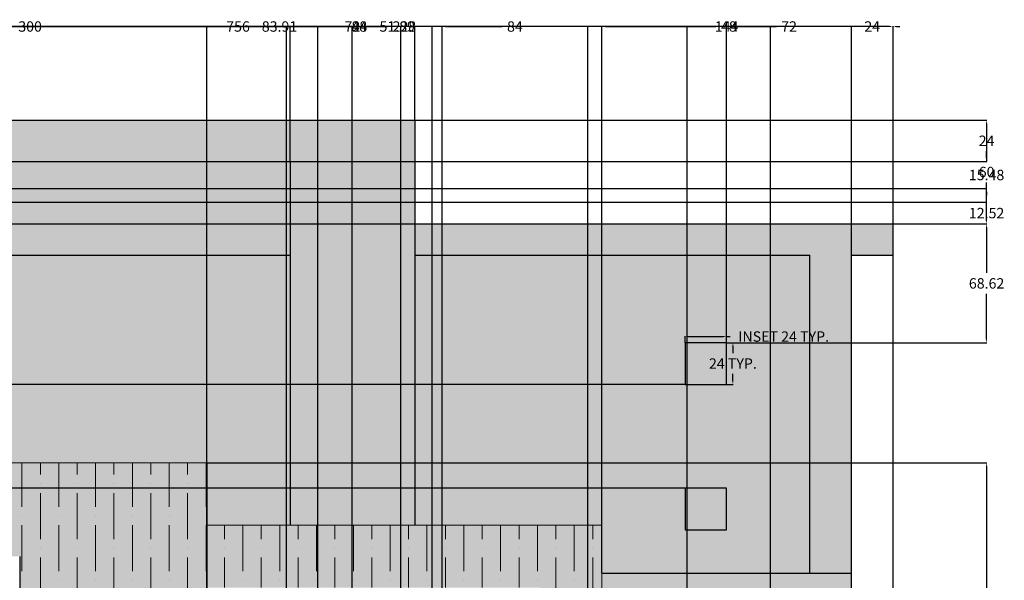
# Model space of a CAD drawing. Units: inches. Extents: x 180 to 1069, y 71 to 1267.
# Tile 8 of 8: x 498 to 1066, y 943 to 1267. Entities that reach past the tile are written whole.
import ezdxf

# ---------------------------------------------------------------- set-up
doc = ezdxf.new("R2010")
doc.units = ezdxf.units.IN
doc.header["$MEASUREMENT"] = 0
for name, color, linetype, lineweight in [('A-ANNO-DIMS', 2, 'Continuous', 18), ('A-ELEV-FRAM', 7, 'Continuous', 25), ('A-WALL', 7, 'Continuous', 30), ('A-WALL-CLAD', 7, 'Continuous', 18), ('A-WALL-SCRN-JNTS-PATT', 8, 'Continuous', 13)]:
    doc.layers.add(name, color=color, linetype=linetype, lineweight=lineweight)
for name, color, linetype, lineweight, true_color in [('A-ELEV-BAND-PATT', 30, 'Continuous', 13, 0xf26722), ('A-ELEV-FRAM-PATT', 53, 'Continuous', 13, 0xefd648), ('A-ELEV-REVL-PATT', 9, 'Continuous', 13, 0xc7c8ca), ('A-ELEV-TRIM-PATT', 7, 'Continuous', 13, 0xffffff), ('A-WALL-PATT', 253, 'Continuous', 13, 0x9f9f8e), ('A-WALL-SCRN-PATT', 251, 'Continuous', 13, 0x636466), ('A-WALL-STUC-PATT', 9, 'Continuous', 13, 0xc7c8ca)]:
    doc.layers.add(name, color=color, linetype=linetype, lineweight=lineweight, true_color=true_color)
doc.styles.get("Standard").update_dxf_attribs({"font": 'arial.ttf'})
doc.dimstyles.get("Standard").update_dxf_attribs({"dimtxt": 6, "dimasz": 2, "dimexe": 0.18, "dimexo": 0.0625, "dimgap": 3, "dimtad": 0, "dimtih": 1, "dimtoh": 1, "dimdec": 0, "dimzin": 0, "dimdsep": 46, "dimlunit": 3, "dimtxsty": 'Standard', "dimcen": 0.09, "dimadec": 0, "dimazin": 0, "dimtfac": 1, "dimtdec": 0, "dimtofl": 0, "dimtmove": 0, "dimatfit": 3, "dimfxl": 1, "dimtolj": 1, "dimtzin": 0, "dimarcsym": 0})

# ---------------------------------------------------------------- blocks, each defined once
blk = doc.blocks.new('FACADE-SQUARE-INSET')
blk.add_lwpolyline([(24, 24), (0, 24), (0, 0), (24, 0)], close=True)
blk = doc.blocks.new('*D6')
at = {"layer": 'A-ANNO-DIMS', "color": 0, "lineweight": -2, "transparency": 16777216}
for p, q in [((882.09, 1080.26), (882.09, 1083.98)), ((884.09, 1083.8), (904.09, 1083.8)), ((906.09, 1080.26), (906.09, 1083.98)), ((906.09, 1083.8), (908.09, 1083.8))]:
    blk.add_line(p, q, dxfattribs=at)
at = {"layer": 'A-ANNO-DIMS', "color": 0, "transparency": 16777216}
for points in [[(884.09, 1084.13), (884.09, 1083.47), (882.09, 1083.8)], [(904.09, 1084.13), (904.09, 1083.47), (906.09, 1083.8)]]:
    blk.add_solid(points, dxfattribs=at)
at = {"layer": 'Defpoints', "color": 0, "transparency": 16777216}
for p in [(882.09, 1080.2), (906.09, 1083.8), (906.09, 1080.2)]:
    blk.add_point(p, dxfattribs=at)
at = {"layer": 'A-ANNO-DIMS', "color": 0, "transparency": 16777216, "insert": (938.98, 1083.8), "char_height": 6, "attachment_point": 5}
blk.add_mtext('\\A1;INSET 24 TYP.', dxfattribs=at)
blk = doc.blocks.new('*D7')
at = {"layer": 'A-ANNO-DIMS', "color": 0, "lineweight": -2, "transparency": 16777216}
for p, q in [((906.15, 1080.2), (909.87, 1080.2)), ((909.69, 1078.2), (909.69, 1074.21)), ((909.69, 1058.2), (909.69, 1062.19)), ((906.15, 1056.2), (909.87, 1056.2))]:
    blk.add_line(p, q, dxfattribs=at)
at = {"layer": 'A-ANNO-DIMS', "color": 0, "transparency": 16777216}
for points in [[(909.35, 1078.2), (910.02, 1078.2), (909.69, 1080.2)], [(909.35, 1058.2), (910.02, 1058.2), (909.69, 1056.2)]]:
    blk.add_solid(points, dxfattribs=at)
at = {"layer": 'Defpoints', "color": 0, "transparency": 16777216}
for p in [(906.09, 1080.2), (906.09, 1056.2), (909.69, 1056.2)]:
    blk.add_point(p, dxfattribs=at)
at = {"layer": 'A-ANNO-DIMS', "color": 0, "transparency": 16777216, "insert": (909.69, 1068.2), "char_height": 6, "attachment_point": 5}
blk.add_mtext('\\A1;24 TYP.', dxfattribs=at)
blk = doc.blocks.new('*D16')
at = {"layer": 'A-ANNO-DIMS', "color": 0, "lineweight": -2, "transparency": 16777216}
for p, q in [((246.09, 1208.88), (246.09, 1263.01)), ((248.09, 1262.83), (614.49, 1262.83)), ((1000.09, 1262.83), (633.69, 1262.83)), ((1002.09, 1148.88), (1002.09, 1263.01))]:
    blk.add_line(p, q, dxfattribs=at)
at = {"layer": 'A-ANNO-DIMS', "color": 0, "transparency": 16777216}
for points in [[(248.09, 1263.16), (248.09, 1262.5), (246.09, 1262.83)], [(1000.09, 1263.16), (1000.09, 1262.5), (1002.09, 1262.83)]]:
    blk.add_solid(points, dxfattribs=at)
at = {"layer": 'Defpoints', "color": 0, "transparency": 16777216}
for p in [(1002.09, 1262.83), (246.09, 1208.82), (1002.09, 1148.82)]:
    blk.add_point(p, dxfattribs=at)
at = {"layer": 'A-ANNO-DIMS', "color": 0, "transparency": 16777216, "insert": (624.09, 1262.83), "char_height": 6, "attachment_point": 5}
blk.add_mtext('\\A1;756', dxfattribs=at)
blk = doc.blocks.new('*D18')
at = {"layer": 'A-ANNO-DIMS', "color": 0, "lineweight": -2, "transparency": 16777216}
for p, q in [((726.15, 1208.82), (1056.28, 1208.82)), ((1056.1, 1206.82), (1056.1, 1184.88)), ((1056.1, 1150.82), (1056.1, 1172.75)), ((1002.15, 1148.82), (1056.28, 1148.82))]:
    blk.add_line(p, q, dxfattribs=at)
at = {"layer": 'A-ANNO-DIMS', "color": 0, "transparency": 16777216}
for points in [[(1055.77, 1206.82), (1056.43, 1206.82), (1056.1, 1208.82)], [(1055.77, 1150.82), (1056.43, 1150.82), (1056.1, 1148.82)]]:
    blk.add_solid(points, dxfattribs=at)
at = {"layer": 'Defpoints', "color": 0, "transparency": 16777216}
for p in [(726.09, 1208.82), (1056.1, 1208.82), (1002.09, 1148.82)]:
    blk.add_point(p, dxfattribs=at)
at = {"layer": 'A-ANNO-DIMS', "color": 0, "transparency": 16777216, "insert": (1056.1, 1178.82), "char_height": 6, "attachment_point": 5}
blk.add_mtext('\\A1;60', dxfattribs=at)
blk = doc.blocks.new('*D21')
at = {"layer": 'A-ANNO-DIMS', "color": 0, "lineweight": -2, "transparency": 16777216}
for p, q in [((354.09, 1184.88), (354.09, 1263.01)), ((356.09, 1262.83), (494.47, 1262.83)), ((652.09, 1262.83), (513.7, 1262.83)), ((654.09, 1184.88), (654.09, 1263.01))]:
    blk.add_line(p, q, dxfattribs=at)
at = {"layer": 'A-ANNO-DIMS', "color": 0, "transparency": 16777216}
for points in [[(356.09, 1263.16), (356.09, 1262.5), (354.09, 1262.83)], [(652.09, 1263.16), (652.09, 1262.5), (654.09, 1262.83)]]:
    blk.add_solid(points, dxfattribs=at)
at = {"layer": 'Defpoints', "color": 0, "transparency": 16777216}
for p in [(654.09, 1262.83), (354.09, 1184.82), (654.09, 1184.82)]:
    blk.add_point(p, dxfattribs=at)
at = {"layer": 'A-ANNO-DIMS', "color": 0, "transparency": 16777216, "insert": (504.09, 1262.83), "char_height": 6, "attachment_point": 5}
blk.add_mtext('\\A1;300', dxfattribs=at)
blk = doc.blocks.new('*D22')
at = {"layer": 'A-ANNO-DIMS', "color": 0, "lineweight": -2, "transparency": 16777216}
for p, q in [((654.09, 1184.88), (654.09, 1263.01)), ((656.09, 1262.83), (682.85, 1262.83)), ((724.09, 1262.83), (697.33, 1262.83)), ((726.09, 1208.88), (726.09, 1263.01))]:
    blk.add_line(p, q, dxfattribs=at)
at = {"layer": 'A-ANNO-DIMS', "color": 0, "transparency": 16777216}
for points in [[(656.09, 1263.16), (656.09, 1262.5), (654.09, 1262.83)], [(724.09, 1263.16), (724.09, 1262.5), (726.09, 1262.83)]]:
    blk.add_solid(points, dxfattribs=at)
at = {"layer": 'Defpoints', "color": 0, "transparency": 16777216}
for p in [(726.09, 1262.83), (726.09, 1208.82), (654.09, 1184.82)]:
    blk.add_point(p, dxfattribs=at)
at = {"layer": 'A-ANNO-DIMS', "color": 0, "transparency": 16777216, "insert": (690.09, 1262.83), "char_height": 6, "attachment_point": 5}
blk.add_mtext('\\A1;72', dxfattribs=at)
blk = doc.blocks.new('*D23')
at = {"layer": 'A-ANNO-DIMS', "color": 0, "lineweight": -2, "transparency": 16777216}
for p, q in [((726.15, 1208.82), (1056.28, 1208.82)), ((1056.1, 1206.82), (1056.1, 1202.83)), ((1056.1, 1186.82), (1056.1, 1190.8)), ((654.15, 1184.82), (1056.28, 1184.82))]:
    blk.add_line(p, q, dxfattribs=at)
at = {"layer": 'A-ANNO-DIMS', "color": 0, "transparency": 16777216}
for points in [[(1055.77, 1206.82), (1056.43, 1206.82), (1056.1, 1208.82)], [(1055.77, 1186.82), (1056.43, 1186.82), (1056.1, 1184.82)]]:
    blk.add_solid(points, dxfattribs=at)
at = {"layer": 'Defpoints', "color": 0, "transparency": 16777216}
for p in [(726.09, 1208.82), (1056.1, 1208.82), (654.09, 1184.82)]:
    blk.add_point(p, dxfattribs=at)
at = {"layer": 'A-ANNO-DIMS', "color": 0, "transparency": 16777216, "insert": (1056.1, 1196.82), "char_height": 6, "attachment_point": 5}
blk.add_mtext('\\A1;24', dxfattribs=at)
blk = doc.blocks.new('*D24')
at = {"layer": 'A-ANNO-DIMS', "color": 0, "lineweight": -2, "transparency": 16777216}
for p, q in [((1056.1, 1186.82), (1056.1, 1188.82)), ((654.15, 1184.82), (1056.28, 1184.82)), ((654.15, 1169.34), (1056.28, 1169.34)), ((1056.1, 1167.34), (1056.1, 1165.34))]:
    blk.add_line(p, q, dxfattribs=at)
at = {"layer": 'A-ANNO-DIMS', "color": 0, "transparency": 16777216}
for points in [[(1055.77, 1186.82), (1056.43, 1186.82), (1056.1, 1184.82)], [(1055.77, 1167.34), (1056.43, 1167.34), (1056.1, 1169.34)]]:
    blk.add_solid(points, dxfattribs=at)
at = {"layer": 'Defpoints', "color": 0, "transparency": 16777216}
for p in [(654.09, 1184.82), (1056.1, 1184.82), (654.09, 1169.34)]:
    blk.add_point(p, dxfattribs=at)
at = {"layer": 'A-ANNO-DIMS', "color": 0, "transparency": 16777216, "insert": (1056.1, 1177.08), "char_height": 6, "attachment_point": 5}
blk.add_mtext('\\A1;15.48', dxfattribs=at)
blk = doc.blocks.new('*D26')
at = {"layer": 'A-ANNO-DIMS', "color": 0, "lineweight": -2, "transparency": 16777216}
for p, q in [((1056.1, 1163.34), (1056.1, 1165.34)), ((654.15, 1161.34), (1056.28, 1161.34)), ((654.15, 1148.82), (1056.28, 1148.82)), ((1056.1, 1146.82), (1056.1, 1144.82))]:
    blk.add_line(p, q, dxfattribs=at)
at = {"layer": 'A-ANNO-DIMS', "color": 0, "transparency": 16777216}
for points in [[(1055.77, 1163.34), (1056.43, 1163.34), (1056.1, 1161.34)], [(1055.77, 1146.82), (1056.43, 1146.82), (1056.1, 1148.82)]]:
    blk.add_solid(points, dxfattribs=at)
at = {"layer": 'Defpoints', "color": 0, "transparency": 16777216}
for p in [(654.09, 1161.34), (1056.1, 1161.34), (654.09, 1148.82)]:
    blk.add_point(p, dxfattribs=at)
at = {"layer": 'A-ANNO-DIMS', "color": 0, "transparency": 16777216, "insert": (1056.1, 1155.08), "char_height": 6, "attachment_point": 5}
blk.add_mtext('\\A1;12.52', dxfattribs=at)
blk = doc.blocks.new('*D40')
at = {"layer": 'A-ANNO-DIMS', "color": 0, "lineweight": -2, "transparency": 16777216}
for p, q in [((652.09, 338.11), (652.09, 1263.01)), ((654.09, 1262.83), (686.8, 1262.83)), ((734.09, 1262.83), (701.38, 1262.83)), ((736.09, 338.11), (736.09, 1263.01))]:
    blk.add_line(p, q, dxfattribs=at)
at = {"layer": 'A-ANNO-DIMS', "color": 0, "transparency": 16777216}
for points in [[(654.09, 1263.16), (654.09, 1262.5), (652.09, 1262.83)], [(734.09, 1263.16), (734.09, 1262.5), (736.09, 1262.83)]]:
    blk.add_solid(points, dxfattribs=at)
at = {"layer": 'Defpoints', "color": 0, "transparency": 16777216}
for p in [(736.09, 1262.83), (652.09, 338.05), (736.09, 338.05)]:
    blk.add_point(p, dxfattribs=at)
at = {"layer": 'A-ANNO-DIMS', "color": 0, "transparency": 16777216, "insert": (694.09, 1262.83), "char_height": 6, "attachment_point": 5}
blk.add_mtext('\\A1;84', dxfattribs=at)
blk = doc.blocks.new('*D42')
at = {"layer": 'A-ANNO-DIMS', "color": 0, "lineweight": -2, "transparency": 16777216}
for p, q in [((670.09, 301.11), (670.09, 1263.01)), ((672.09, 1262.83), (686.66, 1262.83)), ((716.09, 1262.83), (701.51, 1262.83)), ((718.09, 301.11), (718.09, 1263.01))]:
    blk.add_line(p, q, dxfattribs=at)
at = {"layer": 'A-ANNO-DIMS', "color": 0, "transparency": 16777216}
for points in [[(672.09, 1263.16), (672.09, 1262.5), (670.09, 1262.83)], [(716.09, 1263.16), (716.09, 1262.5), (718.09, 1262.83)]]:
    blk.add_solid(points, dxfattribs=at)
at = {"layer": 'Defpoints', "color": 0, "transparency": 16777216}
for p in [(718.09, 1262.83), (670.09, 301.05), (718.09, 301.05)]:
    blk.add_point(p, dxfattribs=at)
at = {"layer": 'A-ANNO-DIMS', "color": 0, "transparency": 16777216, "insert": (694.09, 1262.83), "char_height": 6, "attachment_point": 5}
blk.add_mtext('\\A1;48', dxfattribs=at)
blk = doc.blocks.new('*D44')
at = {"layer": 'A-ANNO-DIMS', "color": 0, "lineweight": -2, "transparency": 16777216}
for p, q in [((606.09, 442.3), (606.09, 1263.01)), ((608.09, 1262.83), (635.5, 1262.83)), ((688, 1262.83), (660.59, 1262.83)), ((690, 442.3), (690, 1263.01))]:
    blk.add_line(p, q, dxfattribs=at)
at = {"layer": 'A-ANNO-DIMS', "color": 0, "transparency": 16777216}
for points in [[(608.09, 1263.16), (608.09, 1262.5), (606.09, 1262.83)], [(688, 1263.16), (688, 1262.5), (690, 1262.83)]]:
    blk.add_solid(points, dxfattribs=at)
at = {"layer": 'Defpoints', "color": 0, "transparency": 16777216}
for p in [(690, 1262.83), (606.09, 442.24), (690, 442.24)]:
    blk.add_point(p, dxfattribs=at)
at = {"layer": 'A-ANNO-DIMS', "color": 0, "transparency": 16777216, "insert": (648.04, 1262.83), "char_height": 6, "attachment_point": 5}
blk.add_mtext('\\A1;83.91', dxfattribs=at)
blk = doc.blocks.new('*D45')
at = {"layer": 'A-ANNO-DIMS', "color": 0, "lineweight": -2, "transparency": 16777216}
for p, q in [((690, 442.3), (690, 1263.01)), ((692, 1262.83), (702.82, 1262.83)), ((739.89, 1262.83), (729.08, 1262.83)), ((741.89, 442.3), (741.89, 1263.01))]:
    blk.add_line(p, q, dxfattribs=at)
at = {"layer": 'A-ANNO-DIMS', "color": 0, "transparency": 16777216}
for points in [[(692, 1263.16), (692, 1262.5), (690, 1262.83)], [(739.89, 1263.16), (739.89, 1262.5), (741.89, 1262.83)]]:
    blk.add_solid(points, dxfattribs=at)
at = {"layer": 'Defpoints', "color": 0, "transparency": 16777216}
for p in [(741.89, 1262.83), (690, 442.24), (741.89, 442.24)]:
    blk.add_point(p, dxfattribs=at)
at = {"layer": 'A-ANNO-DIMS', "color": 0, "transparency": 16777216, "insert": (715.95, 1262.83), "char_height": 6, "attachment_point": 5}
blk.add_mtext('\\A1;51.89', dxfattribs=at)
blk = doc.blocks.new('*D46')
at = {"layer": 'A-ANNO-DIMS', "color": 0, "lineweight": -2, "transparency": 16777216}
for p, q in [((741.89, 442.3), (741.89, 1263.01)), ((743.89, 1262.83), (776.6, 1262.83)), ((823.89, 1262.83), (791.18, 1262.83)), ((825.89, 442.3), (825.89, 1263.01))]:
    blk.add_line(p, q, dxfattribs=at)
at = {"layer": 'A-ANNO-DIMS', "color": 0, "transparency": 16777216}
for points in [[(743.89, 1263.16), (743.89, 1262.5), (741.89, 1262.83)], [(823.89, 1263.16), (823.89, 1262.5), (825.89, 1262.83)]]:
    blk.add_solid(points, dxfattribs=at)
at = {"layer": 'Defpoints', "color": 0, "transparency": 16777216}
for p in [(825.89, 1262.83), (741.89, 442.24), (825.89, 442.24)]:
    blk.add_point(p, dxfattribs=at)
at = {"layer": 'A-ANNO-DIMS', "color": 0, "transparency": 16777216, "insert": (783.89, 1262.83), "char_height": 6, "attachment_point": 5}
blk.add_mtext('\\A1;84', dxfattribs=at)
blk = doc.blocks.new('*D57')
at = {"layer": 'A-ANNO-DIMS', "color": 0, "lineweight": -2, "transparency": 16777216}
for p, q in [((354.09, 1010.88), (354.09, 1263.01)), ((356.09, 1262.83), (470.44, 1262.83)), ((604.09, 1262.83), (489.74, 1262.83)), ((606.09, 1010.88), (606.09, 1263.01))]:
    blk.add_line(p, q, dxfattribs=at)
at = {"layer": 'A-ANNO-DIMS', "color": 0, "transparency": 16777216}
for points in [[(356.09, 1263.16), (356.09, 1262.5), (354.09, 1262.83)], [(604.09, 1263.16), (604.09, 1262.5), (606.09, 1262.83)]]:
    blk.add_solid(points, dxfattribs=at)
at = {"layer": 'Defpoints', "color": 0, "transparency": 16777216}
for p in [(606.09, 1262.83), (354.09, 1010.82), (606.09, 1010.82)]:
    blk.add_point(p, dxfattribs=at)
at = {"layer": 'A-ANNO-DIMS', "color": 0, "transparency": 16777216, "insert": (480.09, 1262.83), "char_height": 6, "attachment_point": 5}
blk.add_mtext('\\A1;252', dxfattribs=at)
blk = doc.blocks.new('*D58')
at = {"layer": 'A-ANNO-DIMS', "color": 0, "lineweight": -2, "transparency": 16777216}
for p, q in [((606.09, 1010.75), (606.09, 74.62)), ((498.09, 956.75), (498.09, 74.62)), ((500.09, 74.8), (542.74, 74.8)), ((604.09, 74.8), (561.44, 74.8))]:
    blk.add_line(p, q, dxfattribs=at)
at = {"layer": 'A-ANNO-DIMS', "color": 0, "transparency": 16777216}
for points in [[(500.09, 75.14), (500.09, 74.47), (498.09, 74.8)], [(604.09, 75.14), (604.09, 74.47), (606.09, 74.8)]]:
    blk.add_solid(points, dxfattribs=at)
at = {"layer": 'Defpoints', "color": 0, "transparency": 16777216}
for p in [(606.09, 1010.82), (498.09, 956.82), (606.09, 74.8)]:
    blk.add_point(p, dxfattribs=at)
at = {"layer": 'A-ANNO-DIMS', "color": 0, "transparency": 16777216, "insert": (552.09, 74.8), "char_height": 6, "attachment_point": 5}
blk.add_mtext('\\A1;108', dxfattribs=at)
blk = doc.blocks.new('*D59')
at = {"layer": 'A-ANNO-DIMS', "color": 0, "lineweight": -2, "transparency": 16777216}
for p, q in [((606.15, 1010.82), (1056.28, 1010.82)), ((1056.1, 1008.82), (1056.1, 728.88)), ((1056.1, 436.82), (1056.1, 716.75)), ((606.15, 434.82), (1056.28, 434.82))]:
    blk.add_line(p, q, dxfattribs=at)
at = {"layer": 'A-ANNO-DIMS', "color": 0, "transparency": 16777216}
for points in [[(1055.77, 1008.82), (1056.43, 1008.82), (1056.1, 1010.82)], [(1055.77, 436.82), (1056.43, 436.82), (1056.1, 434.82)]]:
    blk.add_solid(points, dxfattribs=at)
at = {"layer": 'Defpoints', "color": 0, "transparency": 16777216}
for p in [(606.09, 1010.82), (1056.1, 1010.82), (606.09, 434.82)]:
    blk.add_point(p, dxfattribs=at)
at = {"layer": 'A-ANNO-DIMS', "color": 0, "transparency": 16777216, "insert": (1056.1, 722.82), "char_height": 6, "attachment_point": 5}
blk.add_mtext('\\A1;576', dxfattribs=at)
blk = doc.blocks.new('*D61')
at = {"layer": 'A-ANNO-DIMS', "color": 0, "lineweight": -2, "transparency": 16777216}
for p, q in [((1002.15, 1148.82), (1056.28, 1148.82)), ((1056.1, 1146.82), (1056.1, 1120.57)), ((1056.1, 1082.2), (1056.1, 1108.44)), ((906.15, 1080.2), (1056.28, 1080.2))]:
    blk.add_line(p, q, dxfattribs=at)
at = {"layer": 'A-ANNO-DIMS', "color": 0, "transparency": 16777216}
for points in [[(1055.77, 1146.82), (1056.43, 1146.82), (1056.1, 1148.82)], [(1055.77, 1082.2), (1056.43, 1082.2), (1056.1, 1080.2)]]:
    blk.add_solid(points, dxfattribs=at)
at = {"layer": 'Defpoints', "color": 0, "transparency": 16777216}
for p in [(1002.09, 1148.82), (1056.1, 1148.82), (906.09, 1080.2)]:
    blk.add_point(p, dxfattribs=at)
at = {"layer": 'A-ANNO-DIMS', "color": 0, "transparency": 16777216, "insert": (1056.1, 1114.51), "char_height": 6, "attachment_point": 5}
blk.add_mtext('\\A1;68.62', dxfattribs=at)
blk = doc.blocks.new('*D62')
at = {"layer": 'A-ANNO-DIMS', "color": 0, "lineweight": -2, "transparency": 16777216}
for p, q in [((882.02, 1056.2), (191.89, 1056.2)), ((192.07, 1054.2), (192.07, 1032.26)), ((192.07, 998.2), (192.07, 1020.14)), ((882.02, 996.2), (191.89, 996.2))]:
    blk.add_line(p, q, dxfattribs=at)
at = {"layer": 'A-ANNO-DIMS', "color": 0, "transparency": 16777216}
for points in [[(191.74, 1054.2), (192.41, 1054.2), (192.07, 1056.2)], [(191.74, 998.2), (192.41, 998.2), (192.07, 996.2)]]:
    blk.add_solid(points, dxfattribs=at)
at = {"layer": 'Defpoints', "color": 0, "transparency": 16777216}
for p in [(192.07, 1056.2), (882.09, 1056.2), (882.09, 996.2)]:
    blk.add_point(p, dxfattribs=at)
at = {"layer": 'A-ANNO-DIMS', "color": 0, "transparency": 16777216, "insert": (192.07, 1026.2), "char_height": 6, "attachment_point": 5}
blk.add_mtext('\\A1;60', dxfattribs=at)
blk = doc.blocks.new('*D63')
at = {"layer": 'A-ANNO-DIMS', "color": 0, "lineweight": -2, "transparency": 16777216}
for p, q in [((906.09, 1080.26), (906.09, 1263.01)), ((908.09, 1262.83), (934.85, 1262.83)), ((976.09, 1262.83), (949.33, 1262.83)), ((978.09, 1130.88), (978.09, 1263.01))]:
    blk.add_line(p, q, dxfattribs=at)
at = {"layer": 'A-ANNO-DIMS', "color": 0, "transparency": 16777216}
for points in [[(908.09, 1263.16), (908.09, 1262.5), (906.09, 1262.83)], [(976.09, 1263.16), (976.09, 1262.5), (978.09, 1262.83)]]:
    blk.add_solid(points, dxfattribs=at)
at = {"layer": 'Defpoints', "color": 0, "transparency": 16777216}
for p in [(978.09, 1262.83), (978.09, 1130.82), (906.09, 1080.2)]:
    blk.add_point(p, dxfattribs=at)
at = {"layer": 'A-ANNO-DIMS', "color": 0, "transparency": 16777216, "insert": (942.09, 1262.83), "char_height": 6, "attachment_point": 5}
blk.add_mtext('\\A1;72', dxfattribs=at)
blk = doc.blocks.new('*D74')
at = {"layer": 'A-ANNO-DIMS', "color": 0, "lineweight": -2, "transparency": 16777216}
for p, q in [((976.09, 1262.83), (974.09, 1262.83)), ((978.09, 845.88), (978.09, 1263.01)), ((1002.09, 869.88), (1002.09, 1263.01)), ((1004.09, 1262.83), (1006.09, 1262.83))]:
    blk.add_line(p, q, dxfattribs=at)
at = {"layer": 'A-ANNO-DIMS', "color": 0, "transparency": 16777216}
for points in [[(976.09, 1263.16), (976.09, 1262.5), (978.09, 1262.83)], [(1004.09, 1263.16), (1004.09, 1262.5), (1002.09, 1262.83)]]:
    blk.add_solid(points, dxfattribs=at)
at = {"layer": 'Defpoints', "color": 0, "transparency": 16777216}
for p in [(1002.09, 1262.83), (1002.09, 869.82), (978.09, 845.82)]:
    blk.add_point(p, dxfattribs=at)
at = {"layer": 'A-ANNO-DIMS', "color": 0, "transparency": 16777216, "insert": (990.09, 1262.83), "char_height": 6, "attachment_point": 5}
blk.add_mtext('\\A1;24', dxfattribs=at)
blk = doc.blocks.new('*D75')
at = {"layer": 'A-ANNO-DIMS', "color": 0, "lineweight": -2, "transparency": 16777216}
for p, q in [((606.09, 974.88), (606.09, 1263.01)), ((608.09, 1262.83), (710.4, 1262.83)), ((832.09, 1262.83), (729.77, 1262.83)), ((834.09, 974.88), (834.09, 1263.01))]:
    blk.add_line(p, q, dxfattribs=at)
at = {"layer": 'A-ANNO-DIMS', "color": 0, "transparency": 16777216}
for points in [[(608.09, 1263.16), (608.09, 1262.5), (606.09, 1262.83)], [(832.09, 1263.16), (832.09, 1262.5), (834.09, 1262.83)]]:
    blk.add_solid(points, dxfattribs=at)
at = {"layer": 'Defpoints', "color": 0, "transparency": 16777216}
for p in [(834.09, 1262.83), (606.09, 974.82), (834.09, 974.82)]:
    blk.add_point(p, dxfattribs=at)
at = {"layer": 'A-ANNO-DIMS', "color": 0, "transparency": 16777216, "insert": (720.09, 1262.83), "char_height": 6, "attachment_point": 5}
blk.add_mtext('\\A1;228', dxfattribs=at)
blk = doc.blocks.new('*D76')
at = {"layer": 'A-ANNO-DIMS', "color": 0, "lineweight": -2, "transparency": 16777216}
for p, q in [((834.09, 947.31), (834.09, 1263.01)), ((836.09, 1262.83), (896.75, 1262.83)), ((976.09, 1262.83), (915.42, 1262.83)), ((978.09, 947.31), (978.09, 1263.01))]:
    blk.add_line(p, q, dxfattribs=at)
at = {"layer": 'A-ANNO-DIMS', "color": 0, "transparency": 16777216}
for points in [[(836.09, 1263.16), (836.09, 1262.5), (834.09, 1262.83)], [(976.09, 1263.16), (976.09, 1262.5), (978.09, 1262.83)]]:
    blk.add_solid(points, dxfattribs=at)
at = {"layer": 'Defpoints', "color": 0, "transparency": 16777216}
for p in [(978.09, 1262.83), (834.09, 947.25), (978.09, 947.25)]:
    blk.add_point(p, dxfattribs=at)
at = {"layer": 'A-ANNO-DIMS', "color": 0, "transparency": 16777216, "insert": (906.09, 1262.83), "char_height": 6, "attachment_point": 5}
blk.add_mtext('\\A1;144', dxfattribs=at)
blk = doc.blocks.new('*D77')
at = {"layer": 'A-ANNO-DIMS', "color": 0, "lineweight": -2, "transparency": 16777216}
for p, q in [((883.35, 731.88), (883.35, 1263.01)), ((885.35, 1262.83), (899.93, 1262.83)), ((929.35, 1262.83), (914.78, 1262.83)), ((931.35, 731.88), (931.35, 1263.01))]:
    blk.add_line(p, q, dxfattribs=at)
at = {"layer": 'A-ANNO-DIMS', "color": 0, "transparency": 16777216}
for points in [[(885.35, 1263.16), (885.35, 1262.5), (883.35, 1262.83)], [(929.35, 1263.16), (929.35, 1262.5), (931.35, 1262.83)]]:
    blk.add_solid(points, dxfattribs=at)
at = {"layer": 'Defpoints', "color": 0, "transparency": 16777216}
for p in [(931.35, 1262.83), (883.35, 731.82), (931.35, 731.82)]:
    blk.add_point(p, dxfattribs=at)
at = {"layer": 'A-ANNO-DIMS', "color": 0, "transparency": 16777216, "insert": (907.35, 1262.83), "char_height": 6, "attachment_point": 5}
blk.add_mtext('\\A1;48', dxfattribs=at)

msp = doc.modelspace()

# ---------------------------------------------------------------- hatches: boundary and pattern name
at = {"layer": 'A-ELEV-BAND-PATT'}
h = msp.add_hatch(color=256, dxfattribs=at)
h.dxf.hatch_style = 1
h.paths.add_polyline_path([(1002.0875, 1148.8159), (726.0875, 1148.8159), (726.0875, 1130.8159), (954.0875, 1130.8159), (954.0875, 947.2513), (978.0875, 947.2513), (978.0875, 1130.8159), (1002.0875, 1130.8159)])
h.paths.add_polyline_path([(654.0875, 1148.8159), (354.0875, 1148.8159), (354.0875, 1130.8159), (654.0875, 1130.8159)])
h.paths.add_polyline_path([(606.0875, 434.8159), (246.0875, 434.8159), (246.0875, 416.8159), (606.0875, 416.8159)])
h.paths.add_polyline_path([(978.0875, 845.8159), (726.0875, 845.8159), (726.0875, 791.8159), (978.0875, 791.8159)])
at = {"layer": 'A-ELEV-FRAM-PATT'}
h = msp.add_hatch(color=256, dxfattribs=at)
h.dxf.hatch_style = 1
h.paths.add_polyline_path([(354.0875, 1184.8159), (654.0875, 1184.8159), (654.0875, 974.8159), (726.0875, 974.8159), (726.0875, 1208.8159), (288.0875, 1208.8159), (288.0875, 897.6348), (304.7188, 897.6348), (304.7188, 883.4805), (288.0875, 883.4805), (288.0875, 866.8025), (304.7188, 866.8025), (304.7188, 852.6482), (288.0875, 852.6482), (288.0875, 835.9702), (304.7188, 835.9702), (304.7188, 821.8159), (288.0875, 821.8159), (288.0875, 805.1379), (304.7188, 805.1379), (304.7188, 790.9836), (288.0875, 790.9836), (288.0875, 774.3056), (304.7188, 774.3056), (304.7188, 760.1513), (288.0875, 760.1513), (288.0875, 743.4733), (304.7188, 743.4733), (304.7188, 729.319), (288.0875, 729.319), (288.0875, 434.8159), (354.0875, 434.8159), (354.0875, 456.1177), (317.1892, 456.1177), (317.1892, 516.1177), (354.0875, 516.1177), (354.0875, 924.0304), (317.1892, 924.0304), (317.1892, 984.0304), (354.0875, 984.0304)])
h.paths.add_polyline_path([(1002.0875, 869.8159), (702.0875, 869.8159), (702.0875, 791.8159), (726.0875, 791.8159), (726.0875, 845.8159), (978.0875, 845.8159), (978.0875, 581.8159), (726.0875, 581.8159), (726.0875, 647.8159), (702.0875, 647.8159), (702.0875, 557.8159), (1002.0875, 557.8159)])
h.paths.add_polyline_path([(906.0875, 1080.2003), (882.0875, 1080.2003), (882.0875, 1056.2003), (906.0875, 1056.2003)])
h.paths.add_polyline_path([(906.0875, 996.2003), (882.0875, 996.2003), (882.0875, 972.2003), (906.0875, 972.2003)])
h.paths.add_polyline_path([(636.5273, 869.8159), (612.5273, 869.8159), (612.5273, 845.8159), (636.5273, 845.8159)], flags=17)
h.paths.add_polyline_path([(682.6602, 869.8159), (658.6602, 869.8159), (658.6602, 845.8159), (682.6602, 845.8159)], flags=17)
h.paths.add_polyline_path([(636.5273, 581.8159), (612.5273, 581.8159), (612.5273, 557.8159), (636.5273, 557.8159)], flags=17)
h.paths.add_polyline_path([(682.6602, 581.8159), (658.6602, 581.8159), (658.6602, 557.8159), (682.6602, 557.8159)], flags=17)
h.paths.add_polyline_path([(942.0875, 358.0477), (918.0875, 358.0477), (918.0875, 128.8159), (942.0875, 128.8159)])
h.paths.add_polyline_path([(630.0875, 358.0477), (606.0875, 358.0477), (606.0875, 128.8159), (630.0875, 128.8159)])
at = {"layer": 'A-ELEV-REVL-PATT'}
h = msp.add_hatch(color=256, dxfattribs=at)
h.dxf.hatch_style = 1
h.paths.add_polyline_path([(654.0875, 1161.3367), (654.0875, 1169.3367), (354.0875, 1169.3367), (354.0875, 1161.3367)])
at = {"layer": 'A-ELEV-TRIM-PATT'}
h = msp.add_hatch(color=256, dxfattribs=at)
h.dxf.hatch_style = 1
h.paths.add_polyline_path([(654.0875, 1130.8159), (354.0875, 1130.8159), (354.0875, 1010.8159), (606.0875, 1010.8159), (606.0875, 974.8159), (654.0875, 974.8159)])
h.paths.add_polyline_path([(654.0875, 1161.3367), (354.0875, 1161.3367), (354.0875, 1148.8159), (654.0875, 1148.8159)])
h.paths.add_polyline_path([(654.0875, 1184.8159), (354.0875, 1184.8159), (354.0875, 1169.3367), (654.0875, 1169.3367)])
h.paths.add_polyline_path([(954.0875, 1130.8159), (726.0875, 1130.8159), (726.0875, 974.8159), (834.0875, 974.8159), (834.0875, 947.2513), (954.0875, 947.2513)])
h.paths.add_polyline_path([(882.0875, 1056.2003), (882.0875, 1080.2003), (906.0875, 1080.2003), (906.0875, 1056.2003)], flags=16)
h.paths.add_polyline_path([(882.0875, 996.2003), (906.0875, 996.2003), (906.0875, 972.2003), (882.0875, 972.2003)], flags=16)
at = {"layer": 'A-WALL-PATT'}
h = msp.add_hatch(color=256, dxfattribs=at)
h.dxf.hatch_style = 1
h.paths.add_polyline_path([(978.0875, 947.2513), (834.0875, 947.2513), (834.0875, 869.8159), (978.0875, 869.8159)])
h.paths.add_polyline_path([(978.0875, 557.8159), (834.0875, 557.8159), (834.0875, 473.8159), (978.0875, 473.8159)])
h.paths.add_polyline_path([(960.2423, 791.8159), (606.0875, 791.8159), (606.0875, 647.8159), (883.3511, 647.8159), (883.3511, 731.8159), (907.3511, 731.8159)])
at = {"layer": 'A-WALL-SCRN-JNTS-PATT'}
h = msp.add_hatch(dxfattribs=at)
h.set_pattern_fill('ANSI36', color=256, scale=85, angle=45)
h.paths.add_polyline_path([(606.0875, 938.8159), (798.0875, 938.8159), (798.0875, 869.8159), (834.0875, 869.8159), (834.0875, 974.8159), (606.0875, 974.8159), (606.0875, 1010.8159), (354.0875, 1010.8159), (354.0875, 984.0304), (467.1892, 984.0304), (467.1892, 956.8159), (498.0875, 956.8159), (498.0875, 488.8159), (467.1892, 488.8159), (467.1892, 456.1177), (354.0875, 456.1177), (354.0875, 434.8159), (606.0875, 434.8159), (606.0875, 473.8159), (834.0875, 473.8159), (834.0875, 557.8159), (798.0875, 557.8159), (798.0875, 509.8159), (606.0875, 509.8159)])
at = {"layer": 'A-WALL-SCRN-PATT'}
h = msp.add_hatch(color=256, dxfattribs=at)
h.dxf.hatch_style = 1
h.paths.add_polyline_path([(606.0875, 938.8159), (798.0875, 938.8159), (798.0875, 869.8159), (834.0875, 869.8159), (834.0875, 974.8159), (606.0875, 974.8159), (606.0875, 1010.8159), (354.0875, 1010.8159), (354.0875, 984.0304), (467.1892, 984.0304), (467.1892, 956.8159), (498.0875, 956.8159), (498.0875, 488.8159), (467.1892, 488.8159), (467.1892, 456.1177), (354.0875, 456.1177), (354.0875, 434.8159), (606.0875, 434.8159), (606.0875, 473.8159), (834.0875, 473.8159), (834.0875, 557.8159), (798.0875, 557.8159), (798.0875, 509.8159), (606.0875, 509.8159)])
h.paths.add_polyline_path([(367.1892, 507.1177), (326.1892, 507.1177), (326.1892, 465.1177), (367.1892, 465.1177)])
h.paths.add_polyline_path([(411.1892, 507.1177), (373.1892, 507.1177), (373.1892, 465.1177), (411.1892, 465.1177)], flags=17)
h.paths.add_polyline_path([(458.1892, 507.1177), (417.1892, 507.1177), (417.1892, 465.1177), (458.1892, 465.1177)], flags=17)
h.paths.add_polyline_path([(426.0875, 672.0741), (354.0875, 672.0741), (354.0875, 636.0741), (426.0875, 636.0741)], flags=17)
h.paths.add_polyline_path([(426.0875, 760.0741), (354.0875, 760.0741), (354.0875, 680.0741), (426.0875, 680.0741)], flags=17)
h.paths.add_polyline_path([(426.0875, 804.0741), (354.0875, 804.0741), (354.0875, 768.0741), (426.0875, 768.0741)], flags=17)
h.paths.add_polyline_path([(367.1892, 975.0304), (326.1892, 975.0304), (326.1892, 933.0304), (367.1892, 933.0304)])
h.paths.add_polyline_path([(411.1892, 975.0304), (373.1892, 975.0304), (373.1892, 933.0304), (411.1892, 933.0304)], flags=17)
h.paths.add_polyline_path([(458.1892, 975.0304), (417.1892, 975.0304), (417.1892, 933.0304), (458.1892, 933.0304)], flags=17)
at = {"layer": 'A-WALL-STUC-PATT'}
h = msp.add_hatch(dxfattribs=at)
h.set_pattern_fill('DOTS', color=256, scale=30, angle=135)
h.paths.add_polyline_path([(654.0875, 1184.8159), (354.0875, 1184.8159), (354.0875, 1169.3367), (654.0875, 1169.3367)])
h.paths.add_polyline_path([(654.0875, 1161.3367), (354.0875, 1161.3367), (354.0875, 1148.8159), (654.0875, 1148.8159)])
h = msp.add_hatch(dxfattribs=at)
h.set_pattern_fill('DOTS', color=256, scale=30, angle=135)
h.paths.add_polyline_path([(654.0875, 1130.8159), (354.0875, 1130.8159), (354.0875, 1010.8159), (606.0875, 1010.8159), (606.0875, 974.8159), (654.0875, 974.8159)])
h.paths.add_polyline_path([(954.0875, 1130.8159), (726.0875, 1130.8159), (726.0875, 974.8159), (834.0875, 974.8159), (834.0875, 947.2513), (954.0875, 947.2513)])
h.paths.add_polyline_path([(882.0875, 1080.2003), (906.0875, 1080.2003), (906.0875, 1056.2003), (882.0875, 1056.2003)], flags=16)
h.paths.add_polyline_path([(882.0875, 996.2003), (906.0875, 996.2003), (906.0875, 972.2003), (882.0875, 972.2003)], flags=16)

# ---------------------------------------------------------------- linework, layer by layer
at = {"layer": 'A-ELEV-FRAM'}
for p, q in [((246.0875, 1208.8159), (726.0875, 1208.8159)), ((726.0875, 1208.8159), (726.0875, 974.8159)), ((354.0875, 1184.8159), (654.0875, 1184.8159)), ((654.0875, 1184.8159), (654.0875, 974.8159)), ((354.0875, 1169.3367), (654.0875, 1169.3367)), ((354.0875, 1161.3367), (654.0875, 1161.3367)), ((354.0875, 1148.8159), (654.0875, 1148.8159)), ((726.0875, 1148.8159), (1002.0875, 1148.8159)), ((1002.0875, 1130.8159), (1002.0875, 1148.8159)), ((354.0875, 1130.8159), (654.0875, 1130.8159)), ((978.0875, 1130.8159), (1002.0875, 1130.8159))]:
    msp.add_line(p, q, dxfattribs=at)
at = {"layer": 'A-WALL'}
for p, q in [((726.0875, 1130.8159), (954.0875, 1130.8159)), ((954.0875, 947.2513), (954.0875, 1130.8159)), ((978.0875, 869.8159), (978.0875, 1130.8159)), ((834.0875, 947.2513), (978.0875, 947.2513))]:
    msp.add_line(p, q, dxfattribs=at)
at = {"layer": 'A-WALL-CLAD'}
for p, q in [((354.0875, 1010.8159), (606.0875, 1010.8159)), ((606.0875, 974.8159), (606.0875, 1010.8159)), ((606.0875, 974.8159), (834.0875, 974.8159)), ((834.0875, 974.8159), (834.0875, 869.8159))]:
    msp.add_line(p, q, dxfattribs=at)

# ---------------------------------------------------------------- block references
at = {"layer": 'A-ELEV-FRAM', "rotation": 270.0000000000007}
msp.add_blockref('FACADE-SQUARE-INSET', (882.0875, 1080.2003), dxfattribs=at)
at = {"layer": 'A-ELEV-FRAM'}
msp.add_blockref('FACADE-SQUARE-INSET', (882.0875, 972.2003), dxfattribs=at)

# ---------------------------------------------------------------- dimensions: what is measured, and where the dimension line sits
at = {"layer": 'A-ANNO-DIMS'}
for base, p1, p2, override, picture, middle in [((1002.0875, 1262.8294), (246.0875, 1208.8159), (1002.0875, 1148.8159), {"dimdec": 0, "dimlfac": 1, "dimrnd": 0, "dimzin": 0, "dimdsep": 46, "dimlunit": 2}, '*D16', (624.0875, 1262.8294)), ((654.0875, 1262.8294), (354.0875, 1184.8159), (654.0875, 1184.8159), {"dimdec": 0, "dimlfac": 1, "dimrnd": 0, "dimzin": 0, "dimdsep": 46, "dimlunit": 2}, '*D21', (504.0875, 1262.8294)), ((606.0875, 1262.8294), (354.0875, 1010.8159), (606.0875, 1010.8159), {"dimdec": 0, "dimlfac": 1, "dimrnd": 0, "dimzin": 0, "dimdsep": 46, "dimlunit": 2}, '*D57', (480.0875, 1262.8294)), ((690.001, 1262.8294), (606.0875, 442.2382), (690.001, 442.2382), {"dimdec": 2, "dimlfac": 1, "dimrnd": 0, "dimzin": 0, "dimdsep": 46, "dimlunit": 2}, '*D44', (648.0442, 1262.8294)), ((834.0875, 1262.8294), (606.0875, 974.8159), (834.0875, 974.8159), {"dimdec": 0, "dimlfac": 1, "dimrnd": 0, "dimzin": 0, "dimdsep": 46, "dimlunit": 2}, '*D75', (720.0875, 1262.8294)), ((736.0875, 1262.8294), (652.0875, 338.0477), (736.0875, 338.0477), {"dimdec": 0, "dimlfac": 1, "dimrnd": 0, "dimzin": 0, "dimdsep": 46, "dimlunit": 2}, '*D40', (694.0875, 1262.8294)), ((726.0875, 1262.8294), (654.0875, 1184.8159), (726.0875, 1208.8159), {"dimdec": 0, "dimlfac": 1, "dimrnd": 0, "dimzin": 0, "dimdsep": 46, "dimlunit": 2}, '*D22', (690.0875, 1262.8294)), ((718.0875, 1262.8294), (670.0875, 301.0477), (718.0875, 301.0477), {"dimdec": 0, "dimlfac": 1, "dimrnd": 0, "dimzin": 0, "dimdsep": 46, "dimlunit": 2}, '*D42', (694.0875, 1262.8294)), ((741.8928, 1262.8294), (690.001, 442.2382), (741.8928, 442.2382), {"dimdec": 2, "dimlfac": 1, "dimrnd": 0, "dimzin": 0, "dimdsep": 46, "dimlunit": 2}, '*D45', (715.9469, 1262.8294)), ((825.8928, 1262.8294), (741.8928, 442.2382), (825.8928, 442.2382), {"dimdec": 0, "dimlfac": 1, "dimrnd": 0, "dimzin": 0, "dimdsep": 46, "dimlunit": 2}, '*D46', (783.8928, 1262.8294)), ((978.0875, 1262.8294), (834.0875, 947.2513), (978.0875, 947.2513), {"dimdec": 0, "dimlfac": 1, "dimrnd": 0, "dimzin": 0, "dimdsep": 46, "dimlunit": 2}, '*D76', (906.0875, 1262.8294)), ((931.3511, 1262.8294), (883.3511, 731.8159), (931.3511, 731.8159), {"dimdec": 0, "dimlfac": 1, "dimrnd": 0, "dimzin": 0, "dimdsep": 46, "dimlunit": 2}, '*D77', (907.3511, 1262.8294)), ((978.0875, 1262.8294), (906.0875, 1080.2003), (978.0875, 1130.8159), {"dimdec": 0, "dimlfac": 1, "dimrnd": 0, "dimzin": 0, "dimdsep": 46, "dimlunit": 2}, '*D63', (942.0875, 1262.8294)), ((1002.0875, 1262.8294), (978.0875, 845.8159), (1002.0875, 869.8159), {"dimdec": 0, "dimlfac": 1, "dimrnd": 0, "dimzin": 0, "dimdsep": 46, "dimlunit": 2}, '*D74', (990.0875, 1262.8294)), ((606.0875, 74.8024), (498.0875, 956.8159), (606.0875, 1010.8159), {"dimdec": 0, "dimlfac": 1, "dimrnd": 0, "dimzin": 0, "dimdsep": 46, "dimlunit": 2}, '*D58', (552.0875, 74.8024))]:
    dim = msp.add_linear_dim(base=base, p1=p1, p2=p2, dimstyle='Standard', override=override, dxfattribs=at)
    dim.commit()
    dim.dimension.update_dxf_attribs({"geometry": picture, "text_midpoint": middle})
for base, p1, p2, override, picture, middle in [((1056.101, 1208.8159), (654.0875, 1184.8159), (726.0875, 1208.8159), {"dimdec": 0, "dimlfac": 1, "dimrnd": 0, "dimzin": 0, "dimdsep": 46, "dimlunit": 2}, '*D23', (1056.101, 1196.8159)), ((1056.101, 1208.8159), (1002.0875, 1148.8159), (726.0875, 1208.8159), {"dimdec": 0, "dimlfac": 1, "dimrnd": 0, "dimzin": 0, "dimdsep": 46, "dimlunit": 2}, '*D18', (1056.101, 1178.8159)), ((1056.101, 1184.8159), (654.0875, 1169.3367), (654.0875, 1184.8159), {"dimdec": 2, "dimlfac": 1, "dimrnd": 0, "dimzin": 0, "dimdsep": 46, "dimlunit": 2}, '*D24', (1056.101, 1177.0763)), ((1056.101, 1161.3367), (654.0875, 1148.8159), (654.0875, 1161.3367), {"dimdec": 2, "dimlfac": 1, "dimrnd": 0, "dimzin": 0, "dimdsep": 46, "dimlunit": 2}, '*D26', (1056.101, 1155.0763)), ((1056.101, 1148.8159), (906.0875, 1080.2003), (1002.0875, 1148.8159), {"dimdec": 2, "dimlfac": 1, "dimrnd": 0, "dimzin": 0, "dimdsep": 46, "dimlunit": 2}, '*D61', (1056.101, 1114.5081)), ((192.074, 1056.2003), (882.0875, 996.2003), (882.0875, 1056.2003), {"dimdec": 0, "dimlfac": 1, "dimrnd": 0, "dimzin": 0, "dimdsep": 46, "dimlunit": 2}, '*D62', (192.074, 1026.2003)), ((1056.101, 1010.8159), (606.0875, 434.8159), (606.0875, 1010.8159), {"dimdec": 0, "dimlfac": 1, "dimrnd": 0, "dimzin": 0, "dimdsep": 46, "dimlunit": 2}, '*D59', (1056.101, 722.8159))]:
    dim = msp.add_linear_dim(base=base, p1=p1, p2=p2, angle=90, dimstyle='Standard', override=override, dxfattribs=at)
    dim.commit()
    dim.dimension.update_dxf_attribs({"geometry": picture, "text_midpoint": middle})
for base, p1, p2, angle, text, picture, middle in [((906.0875, 1083.8003), (882.0875, 1080.2003), (906.0875, 1080.2003), 0, 'INSET <> TYP.', '*D6', (938.9797, 1083.8003)), ((909.6875, 1056.2003), (906.0875, 1080.2003), (906.0875, 1056.2003), 270, '<> TYP.', '*D7', (909.6875, 1068.2003))]:
    dim = msp.add_linear_dim(base=base, p1=p1, p2=p2, angle=angle, text=text, dimstyle='Standard', override={"dimdec": 0, "dimlfac": 1, "dimrnd": 0, "dimzin": 0, "dimdsep": 46, "dimlunit": 2}, dxfattribs=at)
    dim.commit()
    dim.dimension.update_dxf_attribs({"geometry": picture, "text_midpoint": middle})

doc.saveas('drawing.dxf')
